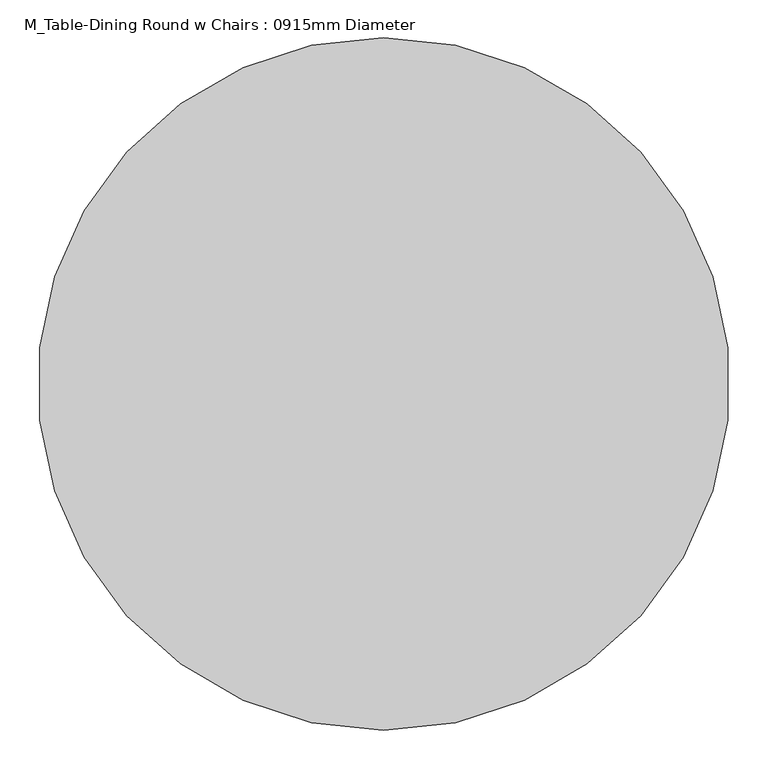
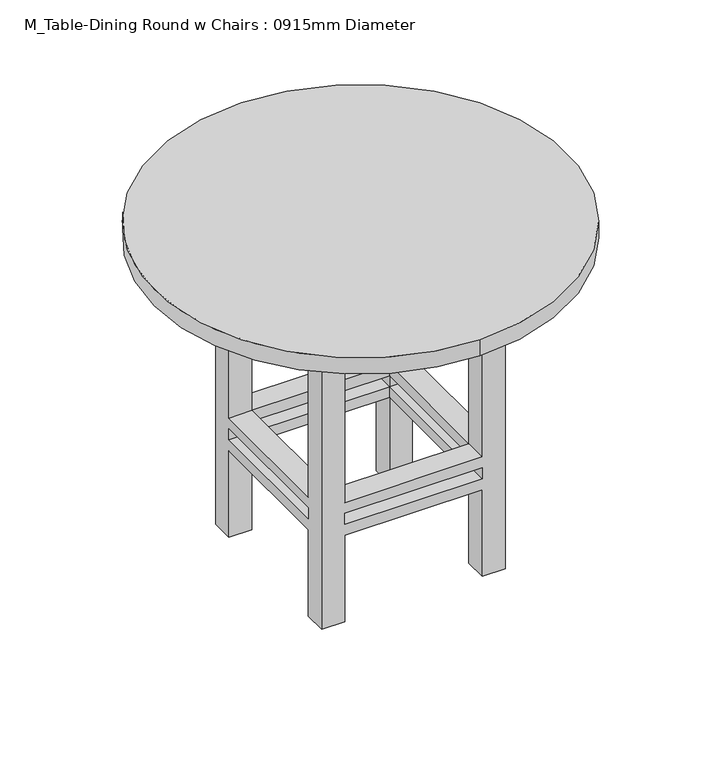
"""IFC4 building model written with IfcOpenShell, lengths in millimetres: furniture geometry, M_Table-Dining Round w Chairs : 0915mm Diameter."""

from ifc_helpers import new_model, si_unit, point, frame, frame_2d, origin, place, context, project, spatial, polyline, circle_curve, trimmed, segment, composite_curve, outline, extrude, faceted_brep, source, transform, mapped, element, save


def m_table_dining_round_w_chairs_0915mm_diameter_5defa876(model_context):
    return source(origin(), model_context, "Body", "SolidModel", [
        faceted_brep([(-48.8680328, 18.4713115, 647.7), (-99.6680328, 18.4713115, 647.7), (-99.6680328, -32.3286885, 647.7), (-48.8680328, -32.3286885, 647.7), (256.2319672, 18.4713115, 647.7), (256.2319672, -32.3286885, 647.7), (307.0319672, -32.3286885, 647.7), (307.0319672, 18.4713115, 647.7), (256.2319672, -388.2286885, 647.7), (307.0319672, -388.2286885, 647.7), (307.0319672, -337.4286885, 647.7), (256.2319672, -337.4286885, 647.7), (-48.8680328, -388.2286885, 647.7), (-48.8680328, -337.4286885, 647.7), (-99.6680328, -337.4286885, 647.7), (-99.6680328, -388.2286885, 647.7), (-48.8680328, 18.4713115, 0.0), (-48.8680328, -32.3286885, 0.0), (-99.6680328, -32.3286885, 0.0), (-99.6680328, 18.4713115, 0.0), (256.2319672, 18.4713115, 0.0), (307.0319672, 18.4713115, 0.0), (307.0319672, -32.3286885, 0.0), (256.2319672, -32.3286885, 0.0), (256.2319672, -388.2286885, 0.0), (256.2319672, -337.4286885, 0.0), (307.0319672, -337.4286885, 0.0), (307.0319672, -388.2286885, 0.0), (-48.8680328, -388.2286885, 0.0), (-99.6680328, -388.2286885, 0.0), (-99.6680328, -337.4286885, 0.0), (-48.8680328, -337.4286885, 0.0), (-48.8680328, 18.4713115, 279.4), (256.2319672, 18.4713115, 279.4), (256.2319672, 18.4713115, 203.2), (-48.8680328, 18.4713115, 203.2), (256.2319672, 18.4713115, 228.6), (256.2319672, 18.4713115, 254.0), (-48.8680328, 18.4713115, 254.0), (-48.8680328, 18.4713115, 228.6), (-99.6680328, -32.3286885, 203.2), (-99.6680328, -337.4286885, 203.2), (-99.6680328, -337.4286885, 279.4), (-99.6680328, -32.3286885, 279.4), (-99.6680328, -32.3286885, 228.6), (-99.6680328, -32.3286885, 254.0), (-99.6680328, -337.4286885, 254.0), (-99.6680328, -337.4286885, 228.6), (-48.8680328, -32.3286885, 279.4), (-48.8680328, -32.3286885, 203.2), (-48.8680328, -32.3286885, 228.6), (-48.8680328, -32.3286885, 254.0), (256.2319672, -32.3286885, 279.4), (256.2319672, -32.3286885, 203.2), (256.2319672, -32.3286885, 228.6), (256.2319672, -32.3286885, 254.0), (307.0319672, -32.3286885, 279.4), (307.0319672, -32.3286885, 203.2), (307.0319672, -32.3286885, 228.6), (307.0319672, -32.3286885, 254.0), (307.0319672, -337.4286885, 279.4), (307.0319672, -337.4286885, 203.2), (307.0319672, -337.4286885, 228.6), (307.0319672, -337.4286885, 254.0), (256.2319672, -388.2286885, 279.4), (-48.8680328, -388.2286885, 279.4), (-48.8680328, -388.2286885, 203.2), (256.2319672, -388.2286885, 203.2), (-48.8680328, -388.2286885, 228.6), (-48.8680328, -388.2286885, 254.0), (256.2319672, -388.2286885, 254.0), (256.2319672, -388.2286885, 228.6), (256.2319672, -337.4286885, 279.4), (256.2319672, -337.4286885, 203.2), (256.2319672, -337.4286885, 228.6), (256.2319672, -337.4286885, 254.0), (-48.8680328, -337.4286885, 279.4), (-48.8680328, -337.4286885, 203.2), (-48.8680328, -337.4286885, 228.6), (-48.8680328, -337.4286885, 254.0)], [[[0, 1, 2, 3]], [[4, 5, 6, 7]], [[8, 9, 10, 11]], [[12, 13, 14, 15]], [[16, 17, 18, 19]], [[20, 21, 22, 23]], [[24, 25, 26, 27]], [[28, 29, 30, 31]], [[1, 0, 32, 33, 4, 7, 21, 20, 34, 35, 16, 19], [36, 37, 38, 39]], [[2, 1, 19, 18, 40, 41, 30, 29, 15, 14, 42, 43], [44, 45, 46, 47]], [[3, 2, 43, 48]], [[18, 17, 49, 40]], [[44, 50, 51, 45]], [[0, 3, 48, 32]], [[17, 16, 35, 49]], [[50, 39, 38, 51]], [[5, 4, 33, 52]], [[20, 23, 53, 34]], [[36, 54, 55, 37]], [[6, 5, 52, 56]], [[23, 22, 57, 53]], [[54, 58, 59, 55]], [[21, 7, 6, 56, 60, 10, 9, 27, 26, 61, 57, 22], [62, 63, 59, 58]], [[27, 9, 8, 64, 65, 12, 15, 29, 28, 66, 67, 24], [68, 69, 70, 71]], [[11, 10, 60, 72]], [[26, 25, 73, 61]], [[62, 74, 75, 63]], [[8, 11, 72, 64]], [[25, 24, 67, 73]], [[74, 71, 70, 75]], [[13, 12, 65, 76]], [[28, 31, 77, 66]], [[68, 78, 79, 69]], [[14, 13, 76, 42]], [[31, 30, 41, 77]], [[78, 47, 46, 79]], [[54, 74, 62, 58]], [[74, 78, 68, 71]], [[78, 50, 44, 47]], [[50, 54, 36, 39]], [[53, 49, 35, 34]], [[49, 77, 41, 40]], [[77, 73, 67, 66]], [[73, 53, 57, 61]], [[74, 54, 53, 73]], [[78, 74, 73, 77]], [[50, 78, 77, 49]], [[54, 50, 49, 53]], [[52, 72, 60, 56]], [[72, 76, 65, 64]], [[76, 48, 43, 42]], [[48, 52, 33, 32]], [[55, 51, 38, 37]], [[51, 79, 46, 45]], [[79, 75, 70, 69]], [[75, 55, 59, 63]], [[72, 52, 55, 75]], [[76, 72, 75, 79]], [[48, 76, 79, 51]], [[52, 48, 51, 55]]]),
        extrude(outline(polyline([(332.4319672, 43.8713115), (332.4319672, -413.6286885), (-125.0680328, -413.6286885), (-125.0680328, 43.8713115), (332.4319672, 43.8713115)]), holes=[polyline([(307.0319672, 18.4713115), (-99.6680328, 18.4713115), (-99.6680328, -388.2286885), (307.0319672, -388.2286885), (307.0319672, 18.4713115)])]), frame((0.0, 0.0, 647.7), z_axis=(0.0, 0.0, 1.0), x_axis=(1.0, 0.0, 0.0)), (0.0, 0.0, 1.0), 76.2),
        extrude(outline(composite_curve([segment(trimmed(circle_curve(frame_2d((103.6819672, -184.8786885)), 457.5), [point((103.6819672, -642.3786885))], [point((103.6819672, 272.6213115))], False, "CARTESIAN"), True, "CONTINUOUS"), segment(trimmed(circle_curve(frame_2d((103.6819672, -184.8786885)), 457.5), [point((103.6819672, 272.6213115))], [point((103.6819672, -642.3786885))], False, "CARTESIAN"), True, "CONTINUOUS")], self_intersect=False)), frame((0.0, 0.0, 723.9), z_axis=(0.0, 0.0, 1.0), x_axis=(1.0, 0.0, 0.0)), (0.0, 0.0, 1.0), 38.1),
    ])


if __name__ == "__main__":
    model = new_model("IFC4")
    model_context = context("Model", 3, world=origin())
    ifc_project = project(units=[si_unit("LENGTHUNIT", "METRE", prefix="MILLI")], contexts=[model_context])
    site = spatial("IfcSite", under=ifc_project)
    building = spatial("IfcBuilding", under=site)
    placement = place(None, origin())
    m_table_dining_round_w_chairs_0915mm_diameter_shape = m_table_dining_round_w_chairs_0915mm_diameter_5defa876(model_context)
    element("IfcFurniture", 1, ObjectType="M_Table-Dining Round w Chairs : 0915mm Diameter", at=placement, inside=building, context=model_context, shape_type="MappedRepresentation", body=[
        mapped(m_table_dining_round_w_chairs_0915mm_diameter_shape, transform((0.0, 0.0, 0.0), x_axis=(1.0, 0.0, 0.0), y_axis=(0.0, 1.0, 0.0), z_axis=(0.0, 0.0, 1.0))),
    ])
    save(model, "model.ifc")

# Revit data of these elements
# Type "M_Table-Dining Round w Chairs : 0915mm Diameter"
#   Radius = 457.5 mm
#   Diameter = 915 mm
#   Height = 762 mm
#   Chairs = 4
#   Base Material = Pine
#   Top Material = Laminate, Linen, Matte
#   Default Elevation = 0
# Element 1 (IfcFurniture, "M_Table-Dining Round w Chairs : 0915mm Diameter")
#   Materials on its faces: "Pine", "Laminate, Linen, Matte"
# Materials
#   "Pine": class "Wood", colour RGB 223 192 134, transparency 0, Description = "Pinus Echinata", Cost = 0
#   "Laminate, Linen, Matte": class "Plastic", colour RGB 249 239 230, transparency 0, Description = "Plastic Laminate - Linen, Matte", Cost = 0
